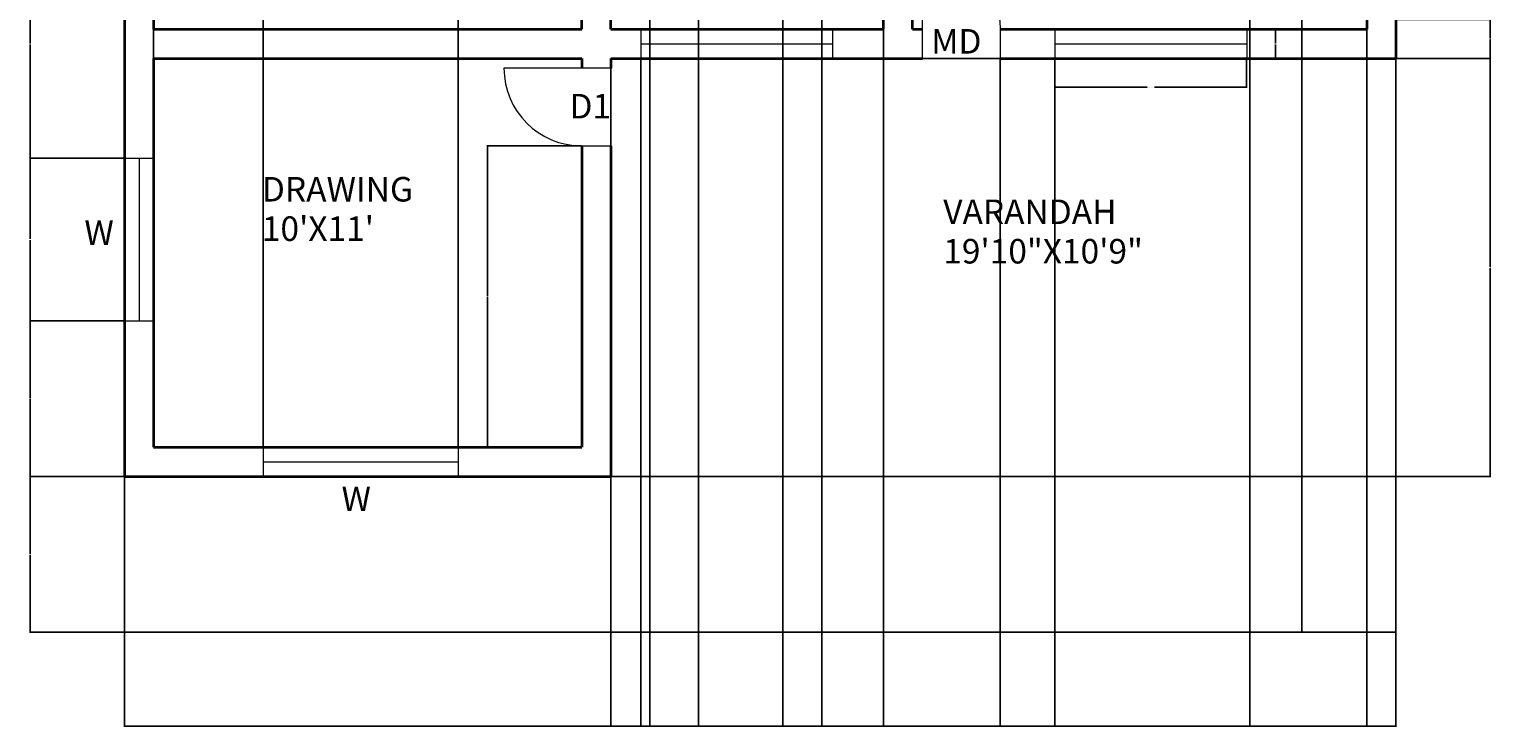
# Model space of a CAD drawing. Units: feet. Extents: x 2075 to 2525, y 1791 to 2414.
# Tile 1 of 3: x 2075 to 2525, y 1791 to 2006. Entities that reach past the tile are written whole.
import ezdxf

# ---------------------------------------------------------------- set-up
doc = ezdxf.new("R2010")
doc.units = ezdxf.units.FT
for name, color, linetype, lineweight in [('A-ANNO-DIMS', 2, 'Continuous', 18), ('A-ANNO-TEXT', 7, 'Continuous', 18), ('A-AREA-IDEN', 7, 'Continuous', 18), ('A-DOOR', 3, 'Continuous', 18), ('A-FLOR', 7, 'Continuous', 25), ('A-GLAZ', 4, 'Continuous', 18), ('A-WALL', 7, 'Continuous', 35)]:
    doc.layers.add(name, color=color, linetype=linetype, lineweight=lineweight)
doc.styles.get("Standard").update_dxf_attribs({"font": 'arial.ttf'})
doc.dimstyles.get("Standard").update_dxf_attribs({"dimtxt": 0.18, "dimasz": 0.18, "dimexe": 0.18, "dimexo": 0.0625, "dimgap": 0.09, "dimtad": 0, "dimtih": 1, "dimtoh": 1, "dimdec": 4, "dimzin": 0, "dimdsep": 46, "dimtxsty": 'Standard', "dimcen": 0.09, "dimadec": 0, "dimazin": 0, "dimtfac": 1, "dimtdec": 4, "dimtofl": 0, "dimtmove": 0, "dimatfit": 3, "dimfxl": 1, "dimtolj": 1, "dimtzin": 0, "dimarcsym": 0})

# ---------------------------------------------------------------- blocks, each defined once
blk = doc.blocks.new('DOOR-SINGLE-SWING')
for p, q in [((24, 0), (24, 33)), ((0, 9), (0, 0))]:
    blk.add_line(p, q)
blk.add_arc((24, 9), 24, 90, 180)
blk = doc.blocks.new('WIN-VERANDAH')
for p, q in [((0, 9), (0, 0)), ((59.14, 9), (59.14, 0)), ((0, 4.5), (59.14, 4.5))]:
    blk.add_line(p, q)
blk = doc.blocks.new('*D11')
at = {"layer": 'A-ANNO-DIMS', "color": 0, "lineweight": -2, "transparency": 16777216}
for p, q in [((2390.79, 1997.27), (2390.79, 1988.28)), ((2449.92, 1997.27), (2449.92, 1988.28)), ((2390.97, 1988.46), (2419.24, 1988.46)), ((2449.74, 1988.46), (2421.47, 1988.46))]:
    blk.add_line(p, q, dxfattribs=at)
at = {"layer": 'A-ANNO-DIMS', "color": 0, "transparency": 16777216}
for points in [[(2390.97, 1988.49), (2390.97, 1988.43), (2390.79, 1988.46)], [(2449.74, 1988.49), (2449.74, 1988.43), (2449.92, 1988.46)]]:
    blk.add_solid(points, dxfattribs=at)
at = {"layer": 'Defpoints', "color": 0, "transparency": 16777216}
for p in [(2390.79, 1997.33), (2449.92, 1997.33), (2449.92, 1988.46)]:
    blk.add_point(p, dxfattribs=at)
at = {"layer": 'A-ANNO-DIMS', "color": 0, "transparency": 16777216, "insert": (2420.36, 1988.46), "char_height": 0.18, "attachment_point": 5}
blk.add_mtext('\\A1;WINDOW 59 TYP.', dxfattribs=at)
blk = doc.blocks.new('*D12')
at = {"layer": 'A-ANNO-DIMS', "color": 0, "lineweight": -2, "transparency": 16777216}
for p, q in [((2449.99, 2006.33), (2458.98, 2006.33)), ((2458.8, 2006.15), (2458.8, 2002.01)), ((2458.8, 1997.51), (2458.8, 2001.65)), ((2449.99, 1997.33), (2458.98, 1997.33))]:
    blk.add_line(p, q, dxfattribs=at)
at = {"layer": 'A-ANNO-DIMS', "color": 0, "transparency": 16777216}
for points in [[(2458.77, 2006.15), (2458.83, 2006.15), (2458.8, 2006.33)], [(2458.77, 1997.51), (2458.83, 1997.51), (2458.8, 1997.33)]]:
    blk.add_solid(points, dxfattribs=at)
at = {"layer": 'Defpoints', "color": 0, "transparency": 16777216}
for p in [(2449.92, 2006.33), (2458.8, 2006.33), (2449.92, 1997.33)]:
    blk.add_point(p, dxfattribs=at)
at = {"layer": 'A-ANNO-DIMS', "color": 0, "transparency": 16777216, "insert": (2458.8, 2001.83), "char_height": 0.18, "attachment_point": 5}
blk.add_mtext('\\A1;9 TYP.', dxfattribs=at)
blk = doc.blocks.new('*D13')
at = {"layer": 'A-ANNO-DIMS', "color": 0, "lineweight": -2, "transparency": 16777216}
for p, q in [((2103.93, 1820.27), (2103.93, 1791.1)), ((2495.93, 1820.27), (2495.93, 1791.1)), ((2104.11, 1791.28), (2299.64, 1791.28)), ((2495.75, 1791.28), (2300.22, 1791.28))]:
    blk.add_line(p, q, dxfattribs=at)
at = {"layer": 'A-ANNO-DIMS', "color": 0, "transparency": 16777216}
for points in [[(2104.11, 1791.31), (2104.11, 1791.25), (2103.93, 1791.28)], [(2495.75, 1791.31), (2495.75, 1791.25), (2495.93, 1791.28)]]:
    blk.add_solid(points, dxfattribs=at)
at = {"layer": 'Defpoints', "color": 0, "transparency": 16777216}
for p in [(2103.93, 1820.33), (2495.93, 1820.33), (2495.93, 1791.28)]:
    blk.add_point(p, dxfattribs=at)
at = {"layer": 'A-ANNO-DIMS', "color": 0, "transparency": 16777216, "insert": (2299.93, 1791.28), "char_height": 0.18, "attachment_point": 5}
blk.add_mtext('\\A1;392', dxfattribs=at)
blk = doc.blocks.new('*D14')
at = {"layer": 'A-ANNO-DIMS', "color": 0, "lineweight": -2, "transparency": 16777216}
for p, q in [((2495.87, 2384.33), (2466.7, 2384.33)), ((2466.88, 2384.15), (2466.88, 2102.51)), ((2466.88, 1820.51), (2466.88, 2102.15)), ((2495.87, 1820.33), (2466.7, 1820.33))]:
    blk.add_line(p, q, dxfattribs=at)
at = {"layer": 'A-ANNO-DIMS', "color": 0, "transparency": 16777216}
for points in [[(2466.85, 2384.15), (2466.91, 2384.15), (2466.88, 2384.33)], [(2466.85, 1820.51), (2466.91, 1820.51), (2466.88, 1820.33)]]:
    blk.add_solid(points, dxfattribs=at)
at = {"layer": 'Defpoints', "color": 0, "transparency": 16777216}
for p in [(2466.88, 2384.33), (2495.93, 2384.33), (2495.93, 1820.33)]:
    blk.add_point(p, dxfattribs=at)
at = {"layer": 'A-ANNO-DIMS', "color": 0, "transparency": 16777216, "insert": (2466.88, 2102.33), "char_height": 0.18, "attachment_point": 5}
blk.add_mtext('\\A1;564', dxfattribs=at)
blk = doc.blocks.new('*D15')
at = {"layer": 'A-ANNO-DIMS', "color": 0, "lineweight": -2, "transparency": 16777216}
for p, q in [((2103.87, 1868.33), (2074.7, 1868.33)), ((2074.88, 1868.15), (2074.88, 1844.51)), ((2074.88, 1820.51), (2074.88, 1844.15)), ((2103.87, 1820.33), (2074.7, 1820.33))]:
    blk.add_line(p, q, dxfattribs=at)
at = {"layer": 'A-ANNO-DIMS', "color": 0, "transparency": 16777216}
for points in [[(2074.85, 1868.15), (2074.91, 1868.15), (2074.88, 1868.33)], [(2074.85, 1820.51), (2074.91, 1820.51), (2074.88, 1820.33)]]:
    blk.add_solid(points, dxfattribs=at)
at = {"layer": 'Defpoints', "color": 0, "transparency": 16777216}
for p in [(2074.88, 1868.33), (2103.93, 1868.33), (2103.93, 1820.33)]:
    blk.add_point(p, dxfattribs=at)
at = {"layer": 'A-ANNO-DIMS', "color": 0, "transparency": 16777216, "insert": (2074.88, 1844.33), "char_height": 0.18, "attachment_point": 5}
blk.add_mtext('\\A1;48', dxfattribs=at)
blk = doc.blocks.new('*D16')
at = {"layer": 'A-ANNO-DIMS', "color": 0, "lineweight": -2, "transparency": 16777216}
for p, q in [((2253.99, 1997.33), (2525.16, 1997.33)), ((2524.98, 1997.15), (2524.98, 1933.01)), ((2524.98, 1868.51), (2524.98, 1932.65)), ((2253.99, 1868.33), (2525.16, 1868.33))]:
    blk.add_line(p, q, dxfattribs=at)
at = {"layer": 'A-ANNO-DIMS', "color": 0, "transparency": 16777216}
for points in [[(2524.95, 1997.15), (2525.01, 1997.15), (2524.98, 1997.33)], [(2524.95, 1868.51), (2525.01, 1868.51), (2524.98, 1868.33)]]:
    blk.add_solid(points, dxfattribs=at)
at = {"layer": 'Defpoints', "color": 0, "transparency": 16777216}
for p in [(2253.93, 1997.33), (2524.98, 1997.33), (2253.93, 1868.33)]:
    blk.add_point(p, dxfattribs=at)
at = {"layer": 'A-ANNO-DIMS', "color": 0, "transparency": 16777216, "insert": (2524.98, 1932.83), "char_height": 0.18, "attachment_point": 5}
blk.add_mtext('\\A1;129', dxfattribs=at)
blk = doc.blocks.new('*D18')
at = {"layer": 'A-ANNO-DIMS', "color": 0, "lineweight": -2, "transparency": 16777216}
for p, q in [((2450.93, 2126.27), (2450.93, 1791.1)), ((2486.93, 2126.27), (2486.93, 1791.1)), ((2451.11, 1791.28), (2468.71, 1791.28)), ((2486.75, 1791.28), (2469.15, 1791.28))]:
    blk.add_line(p, q, dxfattribs=at)
at = {"layer": 'A-ANNO-DIMS', "color": 0, "transparency": 16777216}
for points in [[(2451.11, 1791.31), (2451.11, 1791.25), (2450.93, 1791.28)], [(2486.75, 1791.31), (2486.75, 1791.25), (2486.93, 1791.28)]]:
    blk.add_solid(points, dxfattribs=at)
at = {"layer": 'Defpoints', "color": 0, "transparency": 16777216}
for p in [(2450.93, 2126.33), (2486.93, 2126.33), (2486.93, 1791.28)]:
    blk.add_point(p, dxfattribs=at)
at = {"layer": 'A-ANNO-DIMS', "color": 0, "transparency": 16777216, "insert": (2468.93, 1791.28), "char_height": 0.18, "attachment_point": 5}
blk.add_mtext('\\A1;36', dxfattribs=at)
blk = doc.blocks.new('*D20')
at = {"layer": 'A-ANNO-DIMS', "color": 0, "lineweight": -2, "transparency": 16777216}
for p, q in [((2306.93, 2162.27), (2306.93, 1791.1)), ((2318.93, 2162.27), (2318.93, 1791.1)), ((2307.11, 1791.28), (2312.72, 1791.28)), ((2318.75, 1791.28), (2313.14, 1791.28))]:
    blk.add_line(p, q, dxfattribs=at)
at = {"layer": 'A-ANNO-DIMS', "color": 0, "transparency": 16777216}
for points in [[(2307.11, 1791.31), (2307.11, 1791.25), (2306.93, 1791.28)], [(2318.75, 1791.31), (2318.75, 1791.25), (2318.93, 1791.28)]]:
    blk.add_solid(points, dxfattribs=at)
at = {"layer": 'Defpoints', "color": 0, "transparency": 16777216}
for p in [(2306.93, 2162.33), (2318.93, 2162.33), (2318.93, 1791.28)]:
    blk.add_point(p, dxfattribs=at)
at = {"layer": 'A-ANNO-DIMS', "color": 0, "transparency": 16777216, "insert": (2312.93, 1791.28), "char_height": 0.18, "attachment_point": 5}
blk.add_mtext('\\A1;12', dxfattribs=at)
blk = doc.blocks.new('*D28')
at = {"layer": 'A-ANNO-DIMS', "color": 0, "lineweight": -2, "transparency": 16777216}
for p, q in [((2103.87, 1916.38), (2074.7, 1916.38)), ((2074.88, 1916.2), (2074.88, 1892.54)), ((2074.88, 1868.51), (2074.88, 1892.17)), ((2103.87, 1868.33), (2074.7, 1868.33))]:
    blk.add_line(p, q, dxfattribs=at)
at = {"layer": 'A-ANNO-DIMS', "color": 0, "transparency": 16777216}
for points in [[(2074.85, 1916.2), (2074.91, 1916.2), (2074.88, 1916.38)], [(2074.85, 1868.51), (2074.91, 1868.51), (2074.88, 1868.33)]]:
    blk.add_solid(points, dxfattribs=at)
at = {"layer": 'Defpoints', "color": 0, "transparency": 16777216}
for p in [(2074.88, 1916.38), (2103.93, 1916.38), (2103.93, 1868.33)]:
    blk.add_point(p, dxfattribs=at)
at = {"layer": 'A-ANNO-DIMS', "color": 0, "transparency": 16777216, "insert": (2074.88, 1892.36), "char_height": 0.18, "attachment_point": 5}
blk.add_mtext('\\A1;48.05', dxfattribs=at)
blk = doc.blocks.new('*D29')
at = {"layer": 'A-ANNO-DIMS', "color": 0, "lineweight": -2, "transparency": 16777216}
for p, q in [((2103.87, 1966.51), (2074.7, 1966.51)), ((2074.88, 1966.33), (2074.88, 1941.63)), ((2074.88, 1916.56), (2074.88, 1941.27)), ((2103.87, 1916.38), (2074.7, 1916.38))]:
    blk.add_line(p, q, dxfattribs=at)
at = {"layer": 'A-ANNO-DIMS', "color": 0, "transparency": 16777216}
for points in [[(2074.85, 1966.33), (2074.91, 1966.33), (2074.88, 1966.51)], [(2074.85, 1916.56), (2074.91, 1916.56), (2074.88, 1916.38)]]:
    blk.add_solid(points, dxfattribs=at)
at = {"layer": 'Defpoints', "color": 0, "transparency": 16777216}
for p in [(2074.88, 1966.51), (2103.93, 1966.51), (2103.93, 1916.38)]:
    blk.add_point(p, dxfattribs=at)
at = {"layer": 'A-ANNO-DIMS', "color": 0, "transparency": 16777216, "insert": (2074.88, 1941.45), "char_height": 0.18, "attachment_point": 5}
blk.add_mtext('\\A1;50.13', dxfattribs=at)
blk = doc.blocks.new('*D30')
at = {"layer": 'A-ANNO-DIMS', "color": 0, "lineweight": -2, "transparency": 16777216}
for p, q in [((2103.87, 2037.01), (2074.7, 2037.01)), ((2074.88, 2036.83), (2074.88, 2001.95)), ((2074.88, 1966.69), (2074.88, 2001.58)), ((2103.87, 1966.51), (2074.7, 1966.51))]:
    blk.add_line(p, q, dxfattribs=at)
at = {"layer": 'A-ANNO-DIMS', "color": 0, "transparency": 16777216}
for points in [[(2074.85, 2036.83), (2074.91, 2036.83), (2074.88, 2037.01)], [(2074.85, 1966.69), (2074.91, 1966.69), (2074.88, 1966.51)]]:
    blk.add_solid(points, dxfattribs=at)
at = {"layer": 'Defpoints', "color": 0, "transparency": 16777216}
for p in [(2074.88, 2037.01), (2103.93, 2037.01), (2103.93, 1966.51)]:
    blk.add_point(p, dxfattribs=at)
at = {"layer": 'A-ANNO-DIMS', "color": 0, "transparency": 16777216, "insert": (2074.88, 2001.76), "char_height": 0.18, "attachment_point": 5}
blk.add_mtext('\\A1;70.5', dxfattribs=at)
blk = doc.blocks.new('*D37')
at = {"layer": 'A-ANNO-DIMS', "color": 0, "lineweight": -2, "transparency": 16777216}
for p, q in [((2495.99, 2009.33), (2525.16, 2009.33)), ((2524.98, 2009.15), (2524.98, 2003.51)), ((2524.98, 1997.51), (2524.98, 2003.15)), ((2495.99, 1997.33), (2525.16, 1997.33))]:
    blk.add_line(p, q, dxfattribs=at)
at = {"layer": 'A-ANNO-DIMS', "color": 0, "transparency": 16777216}
for points in [[(2524.95, 2009.15), (2525.01, 2009.15), (2524.98, 2009.33)], [(2524.95, 1997.51), (2525.01, 1997.51), (2524.98, 1997.33)]]:
    blk.add_solid(points, dxfattribs=at)
at = {"layer": 'Defpoints', "color": 0, "transparency": 16777216}
for p in [(2495.93, 2009.33), (2524.98, 2009.33), (2495.93, 1997.33)]:
    blk.add_point(p, dxfattribs=at)
at = {"layer": 'A-ANNO-DIMS', "color": 0, "transparency": 16777216, "insert": (2524.98, 2003.33), "char_height": 0.18, "attachment_point": 5}
blk.add_mtext('\\A1;12', dxfattribs=at)
blk = doc.blocks.new('*D42')
at = {"layer": 'A-ANNO-DIMS', "color": 0, "lineweight": -2, "transparency": 16777216}
for p, q in [((2112.93, 1877.39), (2112.93, 2413.56)), ((2113.11, 2413.38), (2129.33, 2413.38)), ((2146.47, 2413.38), (2130.25, 2413.38)), ((2146.65, 1877.39), (2146.65, 2413.56))]:
    blk.add_line(p, q, dxfattribs=at)
at = {"layer": 'A-ANNO-DIMS', "color": 0, "transparency": 16777216}
for points in [[(2113.11, 2413.41), (2113.11, 2413.35), (2112.93, 2413.38)], [(2146.47, 2413.41), (2146.47, 2413.35), (2146.65, 2413.38)]]:
    blk.add_solid(points, dxfattribs=at)
at = {"layer": 'Defpoints', "color": 0, "transparency": 16777216}
for p in [(2146.65, 2413.38), (2112.93, 1877.33), (2146.65, 1877.33)]:
    blk.add_point(p, dxfattribs=at)
at = {"layer": 'A-ANNO-DIMS', "color": 0, "transparency": 16777216, "insert": (2129.79, 2413.38), "char_height": 0.18, "attachment_point": 5}
blk.add_mtext('\\A1;33.725', dxfattribs=at)
blk = doc.blocks.new('*D43')
at = {"layer": 'A-ANNO-DIMS', "color": 0, "lineweight": -2, "transparency": 16777216}
for p, q in [((2146.65, 1877.39), (2146.65, 2413.56)), ((2146.83, 2413.38), (2176.43, 2413.38)), ((2206.67, 2413.38), (2177.07, 2413.38)), ((2206.85, 1877.39), (2206.85, 2413.56))]:
    blk.add_line(p, q, dxfattribs=at)
at = {"layer": 'A-ANNO-DIMS', "color": 0, "transparency": 16777216}
for points in [[(2146.83, 2413.41), (2146.83, 2413.35), (2146.65, 2413.38)], [(2206.67, 2413.41), (2206.67, 2413.35), (2206.85, 2413.38)]]:
    blk.add_solid(points, dxfattribs=at)
at = {"layer": 'Defpoints', "color": 0, "transparency": 16777216}
for p in [(2206.85, 2413.38), (2146.65, 1877.33), (2206.85, 1877.33)]:
    blk.add_point(p, dxfattribs=at)
at = {"layer": 'A-ANNO-DIMS', "color": 0, "transparency": 16777216, "insert": (2176.75, 2413.38), "char_height": 0.18, "attachment_point": 5}
blk.add_mtext('\\A1;60.2', dxfattribs=at)
blk = doc.blocks.new('*D44')
at = {"layer": 'A-ANNO-DIMS', "color": 0, "lineweight": -2, "transparency": 16777216}
for p, q in [((2253.93, 1997.27), (2253.93, 1791.1)), ((2263.13, 1997.27), (2263.13, 1791.1)), ((2254.11, 1791.28), (2258.27, 1791.28)), ((2262.95, 1791.28), (2258.78, 1791.28))]:
    blk.add_line(p, q, dxfattribs=at)
at = {"layer": 'A-ANNO-DIMS', "color": 0, "transparency": 16777216}
for points in [[(2254.11, 1791.31), (2254.11, 1791.25), (2253.93, 1791.28)], [(2262.95, 1791.31), (2262.95, 1791.25), (2263.13, 1791.28)]]:
    blk.add_solid(points, dxfattribs=at)
at = {"layer": 'Defpoints', "color": 0, "transparency": 16777216}
for p in [(2253.93, 1997.33), (2263.13, 1997.33), (2263.13, 1791.28)]:
    blk.add_point(p, dxfattribs=at)
at = {"layer": 'A-ANNO-DIMS', "color": 0, "transparency": 16777216, "insert": (2258.53, 1791.28), "char_height": 0.18, "attachment_point": 5}
blk.add_mtext('\\A1;9.2', dxfattribs=at)
blk = doc.blocks.new('*D46')
at = {"layer": 'A-ANNO-DIMS', "color": 0, "lineweight": -2, "transparency": 16777216}
for p, q in [((2373.93, 1997.27), (2373.93, 1791.1)), ((2390.79, 1997.27), (2390.79, 1791.1)), ((2374.11, 1791.28), (2381.97, 1791.28)), ((2390.61, 1791.28), (2382.74, 1791.28))]:
    blk.add_line(p, q, dxfattribs=at)
at = {"layer": 'A-ANNO-DIMS', "color": 0, "transparency": 16777216}
for points in [[(2374.11, 1791.31), (2374.11, 1791.25), (2373.93, 1791.28)], [(2390.61, 1791.31), (2390.61, 1791.25), (2390.79, 1791.28)]]:
    blk.add_solid(points, dxfattribs=at)
at = {"layer": 'Defpoints', "color": 0, "transparency": 16777216}
for p in [(2373.93, 1997.33), (2390.79, 1997.33), (2390.79, 1791.28)]:
    blk.add_point(p, dxfattribs=at)
at = {"layer": 'A-ANNO-DIMS', "color": 0, "transparency": 16777216, "insert": (2382.36, 1791.28), "char_height": 0.18, "attachment_point": 5}
blk.add_mtext('\\A1;16.86', dxfattribs=at)
blk = doc.blocks.new('*D48')
at = {"layer": 'A-ANNO-DIMS', "color": 0, "lineweight": -2, "transparency": 16777216}
for p, q in [((2265.93, 2198.27), (2265.93, 1791.1)), ((2280.93, 2198.27), (2280.93, 1791.1)), ((2266.11, 1791.28), (2273.22, 1791.28)), ((2280.75, 1791.28), (2273.64, 1791.28))]:
    blk.add_line(p, q, dxfattribs=at)
at = {"layer": 'A-ANNO-DIMS', "color": 0, "transparency": 16777216}
for points in [[(2266.11, 1791.31), (2266.11, 1791.25), (2265.93, 1791.28)], [(2280.75, 1791.31), (2280.75, 1791.25), (2280.93, 1791.28)]]:
    blk.add_solid(points, dxfattribs=at)
at = {"layer": 'Defpoints', "color": 0, "transparency": 16777216}
for p in [(2265.93, 2198.33), (2280.93, 2198.33), (2280.93, 1791.28)]:
    blk.add_point(p, dxfattribs=at)
at = {"layer": 'A-ANNO-DIMS', "color": 0, "transparency": 16777216, "insert": (2273.43, 1791.28), "char_height": 0.18, "attachment_point": 5}
blk.add_mtext('\\A1;15', dxfattribs=at)
blk = doc.blocks.new('*D51')
at = {"layer": 'A-ANNO-DIMS', "color": 0, "lineweight": -2, "transparency": 16777216}
for p, q in [((2280.93, 2096.27), (2280.93, 1791.1)), ((2337.93, 2096.27), (2337.93, 1791.1)), ((2281.11, 1791.28), (2309.21, 1791.28)), ((2337.75, 1791.28), (2309.65, 1791.28))]:
    blk.add_line(p, q, dxfattribs=at)
at = {"layer": 'A-ANNO-DIMS', "color": 0, "transparency": 16777216}
for points in [[(2281.11, 1791.31), (2281.11, 1791.25), (2280.93, 1791.28)], [(2337.75, 1791.31), (2337.75, 1791.25), (2337.93, 1791.28)]]:
    blk.add_solid(points, dxfattribs=at)
at = {"layer": 'Defpoints', "color": 0, "transparency": 16777216}
for p in [(2280.93, 2096.33), (2337.93, 2096.33), (2337.93, 1791.28)]:
    blk.add_point(p, dxfattribs=at)
at = {"layer": 'A-ANNO-DIMS', "color": 0, "transparency": 16777216, "insert": (2309.43, 1791.28), "char_height": 0.18, "attachment_point": 5}
blk.add_mtext('\\A1;57', dxfattribs=at)
blk = doc.blocks.new('*D53')
at = {"layer": 'A-ANNO-DIMS', "color": 0, "lineweight": -2, "transparency": 16777216}
for p, q in [((2244.87, 1970.33), (2215.7, 1970.33)), ((2215.88, 1970.15), (2215.88, 1924.01)), ((2215.88, 1877.51), (2215.88, 1923.65)), ((2244.87, 1877.33), (2215.7, 1877.33))]:
    blk.add_line(p, q, dxfattribs=at)
at = {"layer": 'A-ANNO-DIMS', "color": 0, "transparency": 16777216}
for points in [[(2215.85, 1970.15), (2215.91, 1970.15), (2215.88, 1970.33)], [(2215.85, 1877.51), (2215.91, 1877.51), (2215.88, 1877.33)]]:
    blk.add_solid(points, dxfattribs=at)
at = {"layer": 'Defpoints', "color": 0, "transparency": 16777216}
for p in [(2215.88, 1970.33), (2244.93, 1970.33), (2244.93, 1877.33)]:
    blk.add_point(p, dxfattribs=at)
at = {"layer": 'A-ANNO-DIMS', "color": 0, "transparency": 16777216, "insert": (2215.88, 1923.83), "char_height": 0.18, "attachment_point": 5}
blk.add_mtext('\\A1;93', dxfattribs=at)

msp = doc.modelspace()

# ---------------------------------------------------------------- linework, layer by layer
at = {"layer": 'A-FLOR'}
for p, q in [((2495.9279, 1997.3311), (2495.9279, 1820.3311)), ((2103.9279, 1877.3311), (2103.9279, 1820.3311)), ((2103.9279, 1820.3311), (2495.9279, 1820.3311))]:
    msp.add_line(p, q, dxfattribs=at)
at = {"layer": 'A-GLAZ'}
for p, q in [((2103.9279, 1966.5149), (2112.9279, 1966.5149)), ((2108.4279, 1966.5149), (2108.4279, 1916.3818)), ((2103.9279, 1916.3818), (2112.9279, 1916.3818)), ((2146.6525, 1877.3311), (2146.6525, 1868.3311)), ((2206.8484, 1877.3311), (2206.8484, 1868.3311)), ((2146.6525, 1872.8311), (2206.8484, 1872.8311))]:
    msp.add_line(p, q, dxfattribs=at)
at = {"layer": 'A-WALL'}
for p, q in [((2103.9279, 2384.3311), (2103.9279, 1868.3311)), ((2103.9279, 2138.3311), (2103.9279, 1868.3311)), ((2112.9279, 2138.3311), (2112.9279, 2006.3311)), ((2244.9279, 2006.3311), (2244.9279, 2111.3311)), ((2346.9279, 2006.3311), (2346.9279, 2105.3311)), ((2253.9279, 2006.3311), (2253.9279, 2096.3311)), ((2337.9279, 2006.3311), (2337.9279, 2096.3311)), ((2112.9279, 2006.3311), (2244.9279, 2006.3311)), ((2253.9279, 2006.3311), (2337.9279, 2006.3311)), ((2346.9279, 2006.3311), (2349.9279, 2006.3311)), ((2373.9279, 2006.3311), (2486.9279, 2006.3311)), ((2486.9279, 2009.3311), (2486.9279, 2006.3311)), ((2495.9279, 2009.3311), (2495.9279, 1997.3311)), ((2103.9279, 1997.3311), (2103.9279, 1877.3311)), ((2112.9279, 1997.3311), (2244.9279, 1997.3311)), ((2112.9279, 1997.3311), (2112.9279, 1877.3311)), ((2244.9279, 1997.3311), (2244.9279, 1994.3311)), ((2253.9279, 1997.3311), (2349.9279, 1997.3311)), ((2253.9279, 1997.3311), (2253.9279, 1994.3311)), ((2373.9279, 1997.3311), (2495.9279, 1997.3311)), ((2244.9279, 1970.3311), (2244.9279, 1877.3311)), ((2253.9279, 1970.3311), (2253.9279, 1868.3311)), ((2112.9279, 1877.3311), (2244.9279, 1877.3311)), ((2103.9279, 1868.3311), (2253.9279, 1868.3311))]:
    msp.add_line(p, q, dxfattribs=at)

# ---------------------------------------------------------------- block references
at = {"layer": 'A-DOOR', "extrusion": (0, 0, -1), "zscale": -1}
msp.add_blockref('DOOR-SINGLE-SWING', (-2373.9278, 1997.331), dxfattribs=at)
at = {"layer": 'A-DOOR', "rotation": 89.99999999999841}
msp.add_blockref('DOOR-SINGLE-SWING', (2253.9281, 1970.3312), dxfattribs=at)
at = {"layer": 'A-GLAZ'}
for p in [(2263.1275, 1997.331), (2390.787, 1997.331)]:
    msp.add_blockref('WIN-VERANDAH', p, dxfattribs=at)

# ---------------------------------------------------------------- texts
at = {"layer": 'A-ANNO-TEXT'}
for s, height, p in [('MD', 7.56937, (2352.673, 1998.8068)), ('D1', 7.56937, (2241.1361, 1978.798)), ('W', 7.5694, (2091.5812, 1939.7564)), ('W', 7.5694, (2170.8514, 1857.6694))]:
    msp.add_text(s, height=height, dxfattribs=at).set_placement(p)
at = {"layer": 'A-AREA-IDEN'}
for s, height, p in [('DRAWING', 7.56937, (2146.2937, 1953.1652)), ('VARANDAH', 7.56937, (2356.3769, 1946.205)), ("10'X11'", 7.56937, (2146.2937, 1941.0057)), ('19\'10"X10\'9"', 7.569372, (2356.3769, 1934.0455))]:
    msp.add_text(s, height=height, dxfattribs=at).set_placement(p)

# ---------------------------------------------------------------- dimensions: what is measured, and where the dimension line sits
at = {"layer": 'A-ANNO-DIMS'}
for base, p1, p2, override, picture, middle in [((2146.6525, 2413.3811), (2112.9279, 1877.3311), (2146.6525, 1877.3311), {"dimdec": 3, "dimlfac": 1, "dimrnd": 0, "dimzin": 0, "dimdsep": 46, "dimlunit": 2}, '*D42', (2129.7902, 2413.3811)), ((2206.8484, 2413.3811), (2146.6525, 1877.3311), (2206.8484, 1877.3311), {"dimdec": 1, "dimlfac": 1, "dimrnd": 0, "dimzin": 0, "dimdsep": 46, "dimlunit": 2}, '*D43', (2176.7504, 2413.3811)), ((2280.9279, 1791.2811), (2265.9279, 2198.3311), (2280.9279, 2198.3311), {"dimdec": 0, "dimlfac": 1, "dimrnd": 0, "dimzin": 0, "dimdsep": 46, "dimlunit": 2}, '*D48', (2273.4279, 1791.2811)), ((2318.9279, 1791.2811), (2306.9279, 2162.3311), (2318.9279, 2162.3311), {"dimdec": 0, "dimlfac": 1, "dimrnd": 0, "dimzin": 0, "dimdsep": 46, "dimlunit": 2}, '*D20', (2312.9279, 1791.2811)), ((2486.9279, 1791.2811), (2450.9279, 2126.3311), (2486.9279, 2126.3311), {"dimdec": 0, "dimlfac": 1, "dimrnd": 0, "dimzin": 0, "dimdsep": 46, "dimlunit": 2}, '*D18', (2468.9279, 1791.2811)), ((2337.9279, 1791.2811), (2280.9279, 2096.3311), (2337.9279, 2096.3311), {"dimdec": 0, "dimlfac": 1, "dimrnd": 0, "dimzin": 0, "dimdsep": 46, "dimlunit": 2}, '*D51', (2309.4279, 1791.2811)), ((2263.1276, 1791.2811), (2253.9279, 1997.3311), (2263.1276, 1997.3311), {"dimdec": 1, "dimlfac": 1, "dimrnd": 0, "dimzin": 0, "dimdsep": 46, "dimlunit": 2}, '*D44', (2258.5277, 1791.2811)), ((2390.7871, 1791.2811), (2373.9279, 1997.3311), (2390.7871, 1997.3311), {"dimdec": 2, "dimlfac": 1, "dimrnd": 0, "dimzin": 0, "dimdsep": 46, "dimlunit": 2}, '*D46', (2382.3575, 1791.2811)), ((2495.9279, 1791.2811), (2103.9279, 1820.3311), (2495.9279, 1820.3311), {"dimdec": 0, "dimlfac": 1, "dimrnd": 0, "dimzin": 0, "dimdsep": 46, "dimlunit": 2}, '*D13', (2299.9279, 1791.2811))]:
    dim = msp.add_linear_dim(base=base, p1=p1, p2=p2, dimstyle='Standard', override=override, dxfattribs=at)
    dim.commit()
    dim.dimension.update_dxf_attribs({"geometry": picture, "text_midpoint": middle})
for base, p1, p2, override, picture, middle in [((2466.8779, 2384.3311), (2495.9279, 1820.3311), (2495.9279, 2384.3311), {"dimdec": 0, "dimlfac": 1, "dimrnd": 0, "dimzin": 0, "dimdsep": 46, "dimlunit": 2}, '*D14', (2466.8779, 2102.3311)), ((2074.8779, 2037.0134), (2103.9279, 1966.5149), (2103.9279, 2037.0134), {"dimdec": 1, "dimlfac": 1, "dimrnd": 0, "dimzin": 0, "dimdsep": 46, "dimlunit": 2}, '*D30', (2074.8779, 2001.7641)), ((2524.9779, 2009.3311), (2495.9279, 1997.3311), (2495.9279, 2009.3311), {"dimdec": 0, "dimlfac": 1, "dimrnd": 0, "dimzin": 0, "dimdsep": 46, "dimlunit": 2}, '*D37', (2524.9779, 2003.3311)), ((2524.9779, 1997.3311), (2253.9279, 1868.3311), (2253.9279, 1997.3311), {"dimdec": 0, "dimlfac": 1, "dimrnd": 0, "dimzin": 0, "dimdsep": 46, "dimlunit": 2}, '*D16', (2524.9779, 1932.8311)), ((2215.8779, 1970.3311), (2244.9279, 1877.3311), (2244.9279, 1970.3311), {"dimdec": 0, "dimlfac": 1, "dimrnd": 0, "dimzin": 0, "dimdsep": 46, "dimlunit": 2}, '*D53', (2215.8779, 1923.8311)), ((2074.8779, 1966.5149), (2103.9279, 1916.3818), (2103.9279, 1966.5149), {"dimdec": 2, "dimlfac": 1, "dimrnd": 0, "dimzin": 0, "dimdsep": 46, "dimlunit": 2}, '*D29', (2074.8779, 1941.4483)), ((2074.8779, 1916.3818), (2103.9279, 1868.3311), (2103.9279, 1916.3818), {"dimdec": 2, "dimlfac": 1, "dimrnd": 0, "dimzin": 0, "dimdsep": 46, "dimlunit": 2}, '*D28', (2074.8779, 1892.3565)), ((2074.8779, 1868.3311), (2103.9279, 1820.3311), (2103.9279, 1868.3311), {"dimdec": 0, "dimlfac": 1, "dimrnd": 0, "dimzin": 0, "dimdsep": 46, "dimlunit": 2}, '*D15', (2074.8779, 1844.3311))]:
    dim = msp.add_linear_dim(base=base, p1=p1, p2=p2, angle=90, dimstyle='Standard', override=override, dxfattribs=at)
    dim.commit()
    dim.dimension.update_dxf_attribs({"geometry": picture, "text_midpoint": middle})
dim = msp.add_linear_dim(base=(2458.7955, 2006.3311), p1=(2449.9249, 1997.3311), p2=(2449.9249, 2006.3311), angle=90, text='<> TYP.', dimstyle='Standard', override={"dimdec": 0, "dimlfac": 1, "dimrnd": 0, "dimzin": 0, "dimdsep": 46, "dimlunit": 2}, dxfattribs=at)
dim.commit()
dim.dimension.update_dxf_attribs({"geometry": '*D12', "text_midpoint": (2458.7955, 2001.8311)})
dim = msp.add_linear_dim(base=(2449.9249, 1988.4605), p1=(2390.7871, 1997.3311), p2=(2449.9249, 1997.3311), text='WINDOW <> TYP.', dimstyle='Standard', override={"dimdec": 0, "dimlfac": 1, "dimrnd": 0, "dimzin": 0, "dimdsep": 46, "dimlunit": 2}, dxfattribs=at)
dim.commit()
dim.dimension.update_dxf_attribs({"geometry": '*D11', "text_midpoint": (2420.356, 1988.4605)})

doc.saveas('drawing.dxf')
